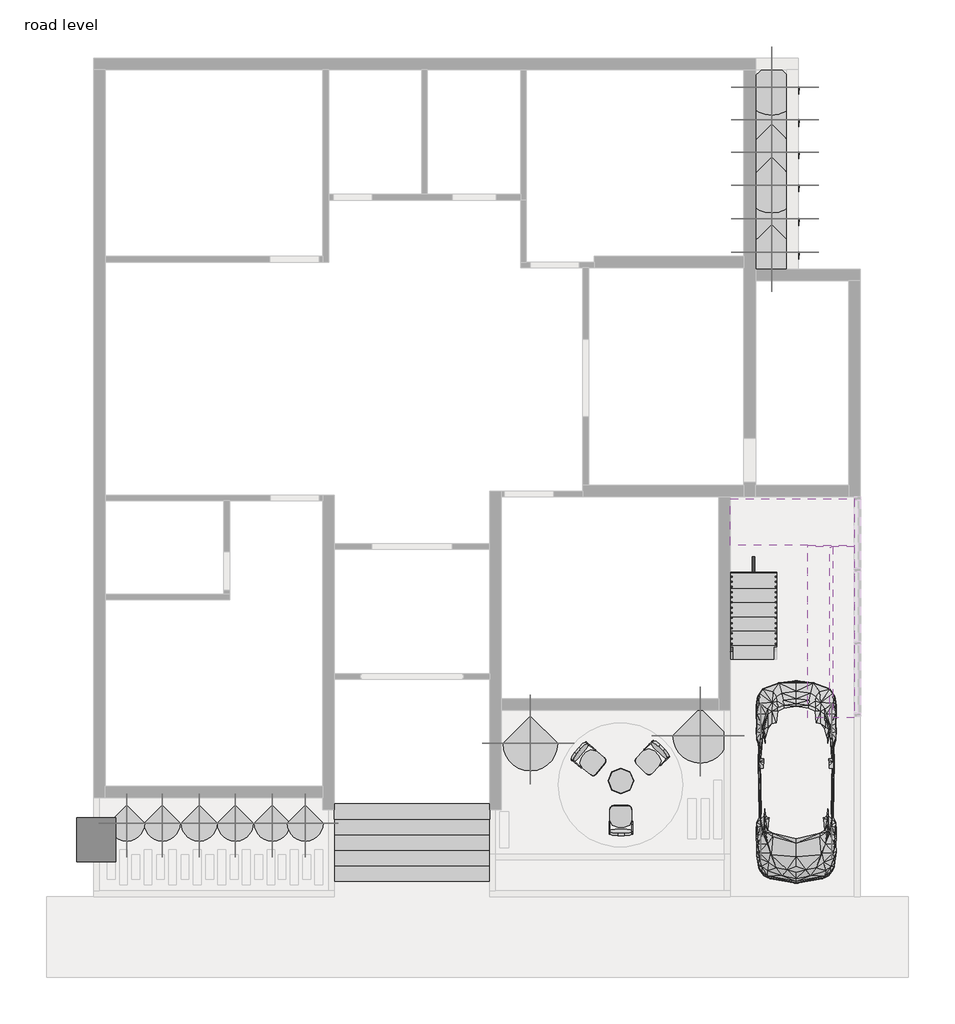
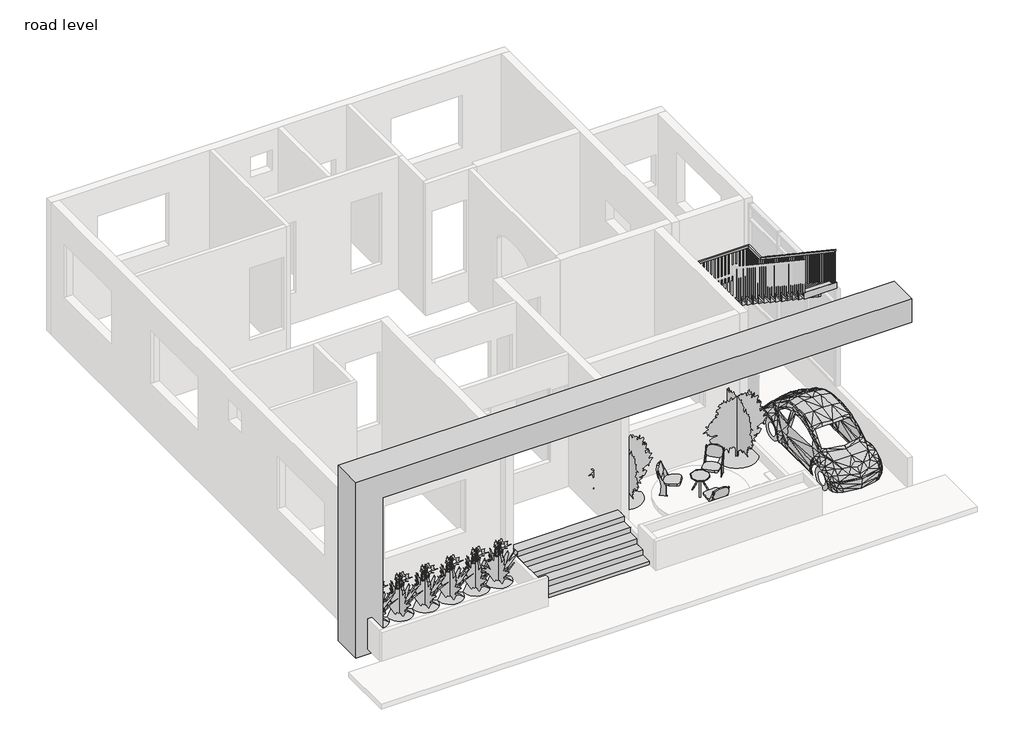
# One storey, part 3 of 3: 14 geographic elements, 6 furniture elements, 2 members, 2 stair flights, 1 proxy, 1 railing, 1 slab.
# Revit data of these elements (continued)
# Type "RPC Plant - Tropical : Japanese Fern - 2.5'" (continued)
#   built-in parameter 1005198 = "{2, 15},{39, RPC-16-G1GK-JAPX-7J4P-Q000-ST1L-LVER-AU},{1, 0},{1, 0},{2, 35},{1, 8},{5, Color},{1, 0},{1, 0},{3, 0.8},{3, 0.8},{3, 0.8},{1, 8},{7, BBoxMin},{1, 0},{1, 0},{1, 0},{1, 0},{1, 0},{1, 8},{7, BBoxMax},{1, 0},{1, 0},{1, 0},{1, 0},{1, 0},{2, 11},{9, RPCTypeId},{1, 0},{1, 0},{39, RPC-16-G1GK-JAPX-7J4P-Q000-ST1L-LVER-AU},{1, 6},{14, RPCPlantHeight},{1, 0},{1, 0},{3, 2.5},{2, 11},{7, keyword},{1, 0},{1, 0},{53, :Geometry:RPC:Japanese Fern:plant:small:japanese fern},{2, 11},{8, category},{1, 0},{1, 0},{17, :Shrubs [General]},{2, 11},{12, LocalizedUID},{1, 0},{1, 0},{13, Japanese Fern},{2, 14},{6, Height},{1, 0},{1, 0},{3, 2.5},{1, 2},{16, Cast Reflections},{1, 0},{1, 0},{1, 0},{1, 2},{12, Cast Shadows},{1, 0},{1, 0},{1, 1},{1, 2},{9, Lock View},{1, 0},{1, 0},{1, 0},{1, 4},{5, ViewC},{1, 0},{1, 0},{1, 0},{2, 11},{20, AdvancedUIDefinition},{1, 0},{1, 0},{0, },{2, 11},{10, AssetLibID},{1, 0},{1, 0},{36, 4D3F6E72-3F99-4203-98E9-AF80B3C7A7A4},{2, 11},{10, BaseSchema},{1, 0},{1, 0},{9, RPCSchema},{2, 11},{12, ExchangeGUID},{1, 0},{1, 0},{0, },{1, 2},{6, Hidden},{1, 0},{1, 0},{1, 0},{1, 4},{11, RPCCategory},{1, 0},{1, 0},{1, 0},{2, 11},{8, RPCImage},{1, 0},{1, 0},{0, },{1, 4},{13, SchemaVersion},{1, 0},{1, 0},{1, 4},{2, 11},{12, UIDefinition},{1, 0},{1, 0},{0, },{2, 11},{6, UIName},{1, 0},{1, 0},{39, RPC-16-G1GK-JAPX-7J4P-Q000-ST1L-LVER-AU},{2, 11},{11, VersionGUID},{1, 0},{1, 0},{9, RPCSchema},{2, 11},{9, assettype},{1, 0},{1, 0},{11, RPCGeometry},{2, 11},{11, description},{1, 0},{1, 0},{0, },{2, 11},{9, localname},{1, 0},{1, 0},{3, RPC},{2, 11},{9, localtype},{1, 0},{1, 0},{3, RPC},{1, 4},{8, revision},{1, 0},{1, 0},{1, 1},{2, 11},{9, thumbnail},{1, 0},{1, 0},{0, },{1, 4},{7, version},{1, 0},{1, 0},{1, 1},{1, 2},{20, RPC_Cast Reflections},{1, 0},{1, 0},{1, 1},{1, 2},{16, RPC_Cast Shadows},{1, 0},{1, 0},{1, 1},{1, 2},{13, RPC_Lock View},{1, 0},{1, 0},{1, 0},{1, 4},{9, RPC_ViewC},{1, 0},{1, 0},{1, 0},{21, assetlibrary_base.fbx},{1, 5},"
#   built-in parameter 1005195 = "RPC-16-G1GK-JAPX-7J4P-Q000-ST1L-LVER-AU"
#   Type Comments = "Japanese Fern"
#   Assembly Code = "G2050500"
#   Height = 4' - 0"
#   Default Elevation = 0
# Type "RPC Plant - Tropical : Jungle Flame - 3'"
#   built-in parameter 1005198 = "{2, 15},{39, RPC-16-FUVJ-JWG0-MWGK-8000-ST1L-LVER-AU},{1, 0},{1, 0},{2, 35},{1, 8},{5, Color},{1, 0},{1, 0},{3, 0.8},{3, 0.8},{3, 0.8},{1, 8},{7, BBoxMin},{1, 0},{1, 0},{1, 0},{1, 0},{1, 0},{1, 8},{7, BBoxMax},{1, 0},{1, 0},{1, 0},{1, 0},{1, 0},{2, 11},{9, RPCTypeId},{1, 0},{1, 0},{39, RPC-16-FUVJ-JWG0-MWGK-8000-ST1L-LVER-AU},{1, 6},{14, RPCPlantHeight},{1, 0},{1, 0},{1, 3},{2, 11},{7, keyword},{1, 0},{1, 0},{90, :Geometry:RPC:Jungle Flame:ixora macrothyrsa:jungle flame:bush:shrub:plant:flower:tropical},{2, 11},{8, category},{1, 0},{1, 0},{17, :Shrubs [General]},{2, 11},{12, LocalizedUID},{1, 0},{1, 0},{12, Jungle Flame},{2, 14},{6, Height},{1, 0},{1, 0},{1, 3},{1, 2},{16, Cast Reflections},{1, 0},{1, 0},{1, 0},{1, 2},{12, Cast Shadows},{1, 0},{1, 0},{1, 1},{1, 2},{9, Lock View},{1, 0},{1, 0},{1, 0},{1, 4},{5, ViewC},{1, 0},{1, 0},{1, 0},{2, 11},{20, AdvancedUIDefinition},{1, 0},{1, 0},{0, },{2, 11},{10, AssetLibID},{1, 0},{1, 0},{36, 4D3F6E72-3F99-4203-98E9-AF80B3C7A7A4},{2, 11},{10, BaseSchema},{1, 0},{1, 0},{9, RPCSchema},{2, 11},{12, ExchangeGUID},{1, 0},{1, 0},{0, },{1, 2},{6, Hidden},{1, 0},{1, 0},{1, 0},{1, 4},{11, RPCCategory},{1, 0},{1, 0},{1, 0},{2, 11},{8, RPCImage},{1, 0},{1, 0},{0, },{1, 4},{13, SchemaVersion},{1, 0},{1, 0},{1, 4},{2, 11},{12, UIDefinition},{1, 0},{1, 0},{0, },{2, 11},{6, UIName},{1, 0},{1, 0},{39, RPC-16-FUVJ-JWG0-MWGK-8000-ST1L-LVER-AU},{2, 11},{11, VersionGUID},{1, 0},{1, 0},{9, RPCSchema},{2, 11},{9, assettype},{1, 0},{1, 0},{11, RPCGeometry},{2, 11},{11, description},{1, 0},{1, 0},{0, },{2, 11},{9, localname},{1, 0},{1, 0},{3, RPC},{2, 11},{9, localtype},{1, 0},{1, 0},{3, RPC},{1, 4},{8, revision},{1, 0},{1, 0},{1, 1},{2, 11},{9, thumbnail},{1, 0},{1, 0},{0, },{1, 4},{7, version},{1, 0},{1, 0},{1, 1},{1, 2},{20, RPC_Cast Reflections},{1, 0},{1, 0},{1, 1},{1, 2},{16, RPC_Cast Shadows},{1, 0},{1, 0},{1, 1},{1, 2},{13, RPC_Lock View},{1, 0},{1, 0},{1, 0},{1, 4},{9, RPC_ViewC},{1, 0},{1, 0},{1, 0},{21, assetlibrary_base.fbx},{1, 5},"
#   built-in parameter 1005195 = "RPC-16-FUVJ-JWG0-MWGK-8000-ST1L-LVER-AU"
#   Type Comments = "Jungle Flame"
#   Assembly Code = "G2050500"
#   Height = 6' - 0"
#   Default Elevation = 0
# Type "Handrail - Rectangular"
#   Assembly Code = "C2010400"
#   built-in parameter 1008612 = 0.0416667 (stored number, unit not read)
#   built-in parameter 1008611 = 0.0416667 (stored number, unit not read)
#   built-in parameter 1008609 = 0.333333 (stored number, unit not read)
#   built-in parameter 1008604 = 0.166667 (stored number, unit not read)
#   built-in parameter 1008603 = 0.166667 (stored number, unit not read)
#   Railing Height = 3' - 0"
#   built-in parameter 1008630 = 2
#   built-in parameter 1008610 = 2
#   built-in parameter 1008618 = Baluster - Square : 3/4"
# Element 1 (IfcBuildingElementProxy, "RPC Beetle : RPC Beetle")
#   Phase Created = New Construction
# Element 2 (IfcFurniture, "Casework 1 : Casework 1")
#   Phase Created = New Construction
# Element 3 (IfcFurniture, "Casework 2 : Casework 2")
#   Phase Created = New Construction
#   Materials on its faces: "Clad - White"
# Elements 4, 5, 6 (IfcFurniture, "Seating-Auditorium : 18\" x 24\" x 30\"")
#   Phase Created = New Construction
#   Materials on its faces: "Steel, Paint Finish, Dark Gray, Matte", "Linen, Beige"
# Element 7 (IfcFurniture, "Table-Trio End : 20\" Diameter")
#   Phase Created = New Construction
#   Materials on its faces: "Wood - Birch", "Laminate - Ivory,Matte"
# Elements 8, 9, 10, 11, 12, 13 (IfcGeographicElement, "RPC Plant - Tropical")
#   Phase Created = New Construction
# Elements 14, 15, 16, 17, 18, 19 (IfcGeographicElement, "RPC Plant - Tropical : Japanese Fern - 2.5'")
#   Phase Created = New Construction
# Elements 20, 21 (IfcGeographicElement, "RPC Plant - Tropical : Jungle Flame - 3'")
#   Phase Created = New Construction
# Elements 22, 23 (IfcMember, "Carriage - 2\" Width")
#   Phase Created = New Construction
# Element 24 (IfcRailing, "Handrail - Rectangular")
#   Phase Created = New Construction
# Element 25 (IfcSlab, "Non-Monolithic Landing")
#   Phase Created = New Construction
# Elements 26, 27 (IfcStairFlight, "2\" Tread 1\" Nosing 1/4\" Riser")
#   Phase Created = New Construction
# Materials
#   "Linen, Beige": class "Textile", colour RGB 249 239 230, transparency 0, Description = "Linen, beige", Cost = 0
#   "Steel, Paint Finish, Dark Gray, Matte": class "Metal", colour RGB 0 0 0, transparency 0, Description = "Steel, paint finish, dark gray, matte", Cost = 0
#   "Wood - Birch": colour RGB 230 196 162, transparency 0
#   "Laminate - Ivory,Matte": colour RGB 127 127 127, transparency 0
#   "Clad - White": class "Wood", colour RGB 242 242 238, transparency 0, Cost = 0
